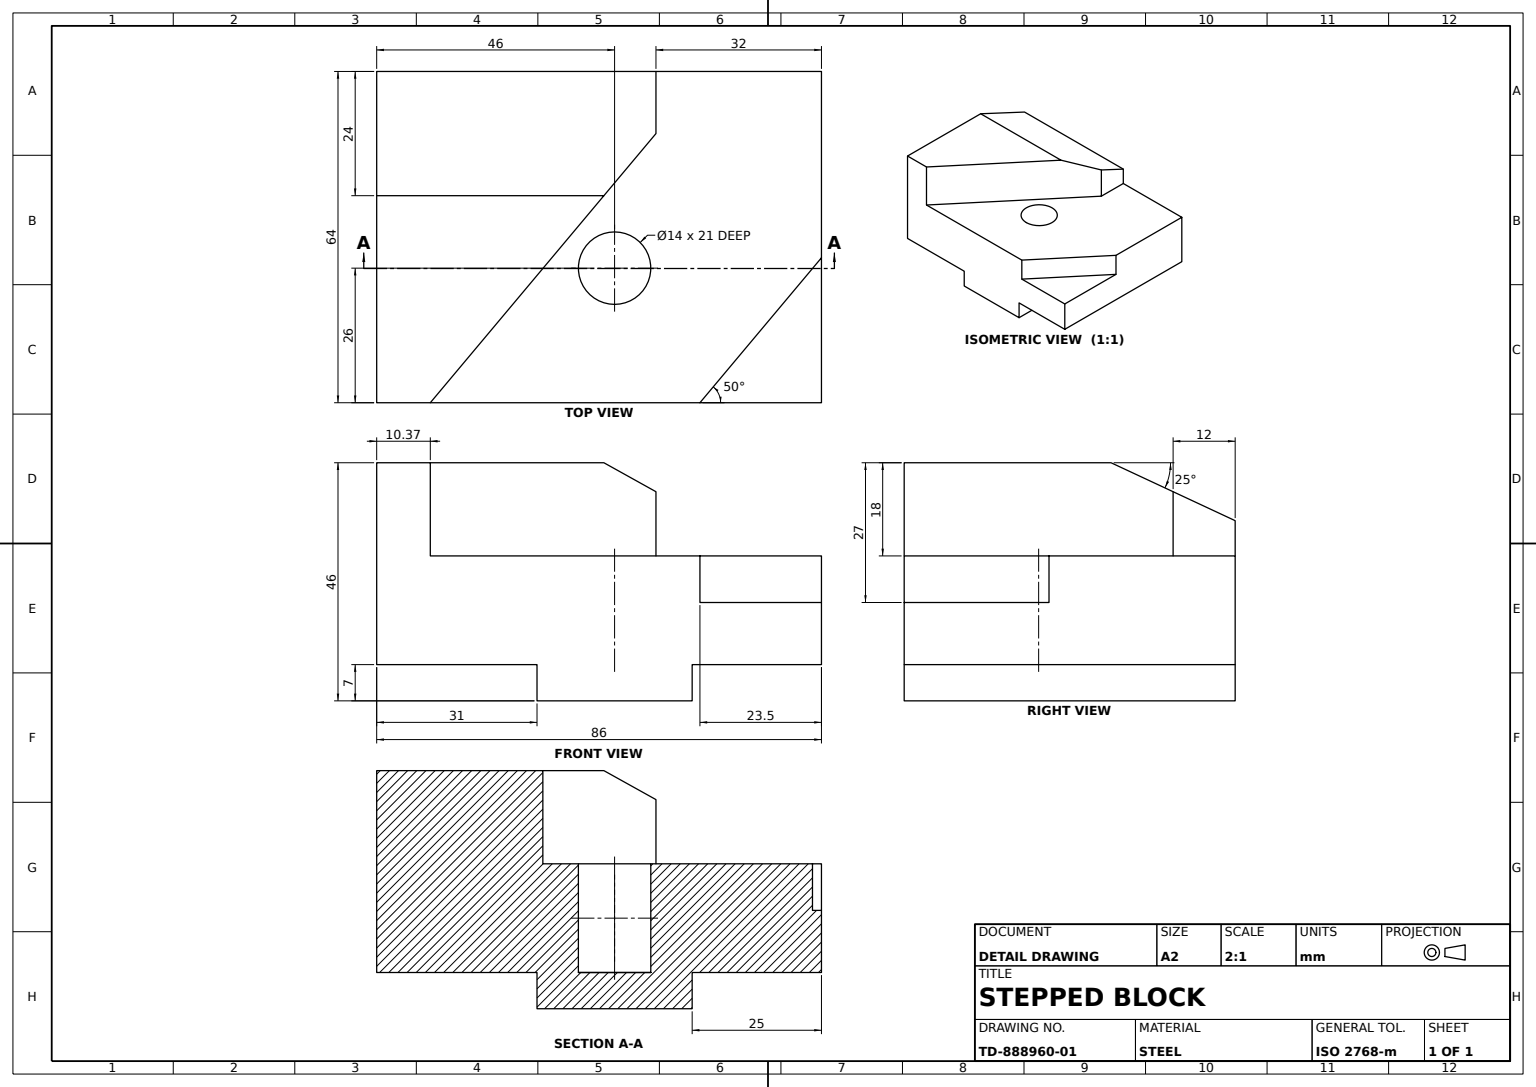
SolidWorks part; units mm, degrees
material "Plain Carbon Steel"
ref_plane "Front Plane" through (0, 0, 0) normal (0, 0, 1) x (1, 0, 0)
ref_plane "Top Plane" through (0, 0, 0) normal (0, 1, 0) x (1, 0, 0)
ref_plane "Right Plane" through (0, 0, 0) normal (1, 0, 0) x (0, 0, -1)
sketch "Base Block Sketch" plane through (0, 0, 0) normal (0, 1, 0) x (1, 0, 0)
  line L1 (-43, -32) -> (43, -32)
  line L2 (-43, -32) -> (-43, 32)
  line L3 (-43, 32) -> (43, 32)
  line L4 (43, -32) -> (43, 32)
  line L5 (-43, -32) -> (43, 32) construction
  line L6 (-43, 32) -> (43, -32) construction
  point P0 (0, 0)
  dimension "D1" = 86
  dimension "D2" = 64
extrude "Base Block 86x64x39" add sketch "Base Block Sketch" along normal blind 39
sketch "Angled Side Cut Sketch" plane through (43, 0, 0) normal (1, 0, 0) x (0, 0, -1)
  line L0 (8, 39) -> (32, 27.8086)
  line L1 (-32, 39) -> (32, 39) construction
  line L2 (32, 39) -> (32, 0) construction
  line L3 (8, 39) -> (32, 39)
  line L4 (32, 39) -> (32, 27.8086)
  dimension "D1" = 25
  dimension "D2" = 24
extrude "Angled Side Cut 25deg" cut sketch "Angled Side Cut Sketch" against normal blind 129
sketch "Top Step Cut Sketch" plane through (0, 39, 0) normal (0, 1, 0) x (1, 0, 0)
  line L0 (11, 32) -> (11, 20)
  line L1 (-43, 32) -> (43, 32) construction
  line L2 (11, 20) -> (-32.6332, -32)
  line L3 (-43, -32) -> (43, -32) construction
  line L7 (43, 8) -> (43, 32) construction
  line L9 (19.5027, -32) -> (43, -3.997)
  line L13 (43, -32) -> (43, 8) construction
  line L15 (43, 8) -> (-43, 8) construction
  line L16 (11, 32) -> (43, 32)
  line L18 (-32.6332, -32) -> (19.5027, -32)
  line L19 (43, 32) -> (43, -3.997)
  circle A0 centre (3, -6) radius 7
  dimension "D6" = 14
  dimension "D1" = 12
  dimension "D2" = 32
  dimension "D3" = 23.4973
  dimension "D4" = 40
  dimension "D5" = 26
  dimension "D7" = 75.6332
  dimension "D8" = 11.997
extrude "Top Step Cut" cut sketch "Top Step Cut Sketch" against normal blind 18
sketch "Corner Bevel Cut Sketch" plane through (0, 39, 0) normal (0, 1, 0) x (1, 0, 0)
  line L0 (43, -3.997) -> (19.5027, -32)
  line L1 (19.5027, -32) -> (43, -32)
  line L2 (43, -32) -> (43, -3.997)
extrude "Corner Bevel Cut" cut sketch "Corner Bevel Cut Sketch" against normal blind 27
sketch "Through Hole Sketch" plane through (0, 39, 0) normal (0, 1, 0) x (1, 0, 0)
  circle A0 centre (3, -6) radius 7
  dimension "D1" = 14
extrude "Through Hole" cut sketch "Through Hole Sketch" against normal blind 97
sketch "Guide Tongue Sketch" plane through (0, 0, 32) normal (0, 0, 1) x (1, 0, 0)
  line L0 (-43, 0) -> (43, 0) construction
  line L1 (-12, 0) -> (18, 0)
  line L2 (-12, 0) -> (-12, -7)
  line L3 (-12, -7) -> (18, -7)
  line L4 (18, 0) -> (18, -7)
  line L5 (43, 12) -> (43, 0) construction
  point P6 (-12, -3.5)
  dimension "D1" = 31
  dimension "D2" = 25
  dimension "D3" = 7
extrude "Guide Tongue" add sketch "Guide Tongue Sketch" against normal blind 64
